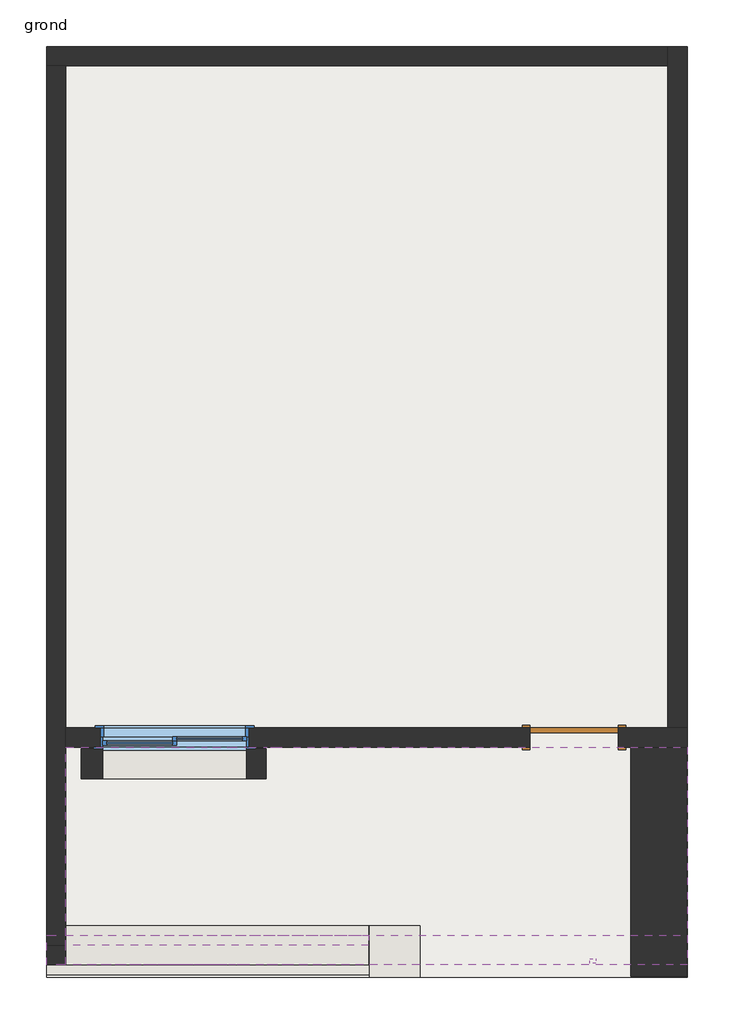
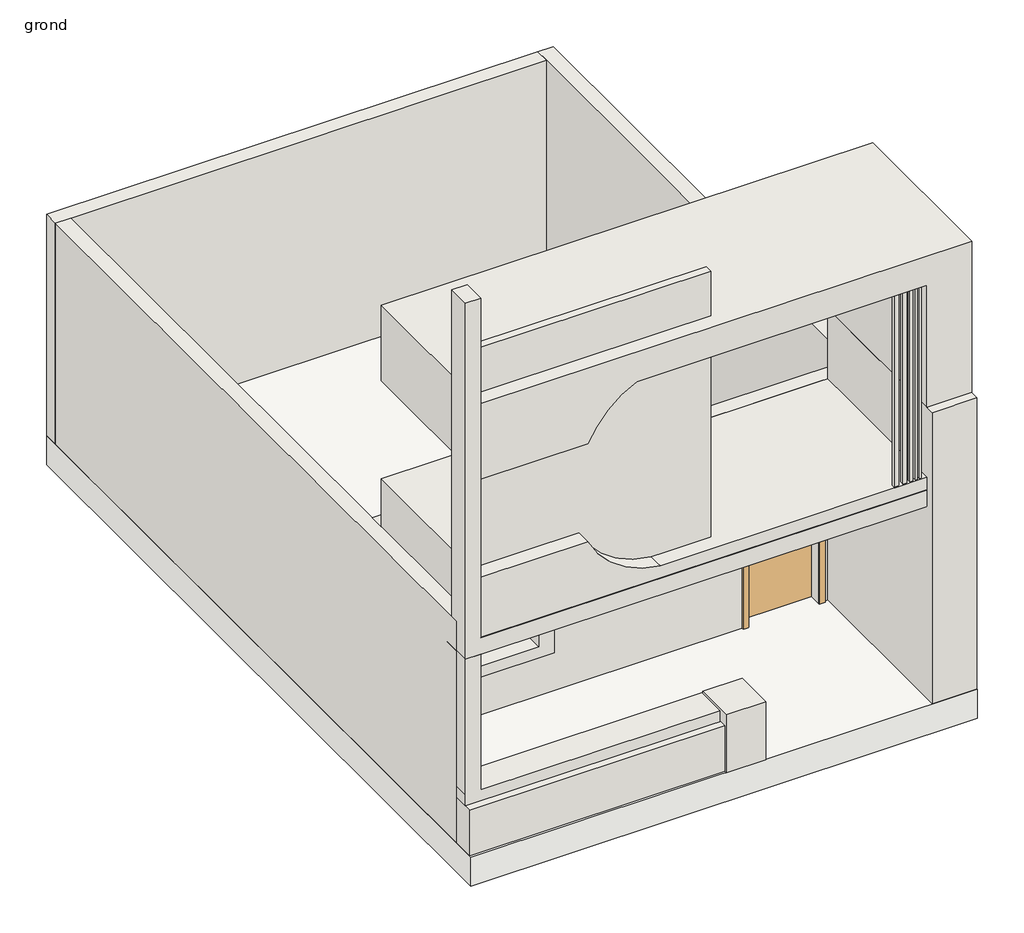
# One storey: 14 walls, 1 door, 1 slab, 1 window.
"""IFC4 building model written with IfcOpenShell, lengths in millimetres."""

from ifc_helpers import new_model, si_unit, frame, origin, origin_with_axes, place, context, project, spatial, polyline, outline, extrude, faceted_brep, transform, mapped, element, save
from components import m_single_flush_0915_x_2134mm_6a9e8738, walls_1_walls_1_6260b2a2, walls_10_walls_10_b49e789a, walls_2_walls_2_db01f069, walls_3_walls_3_21c244ff, walls_4_walls_4_0e46dea8, walls_5_walls_5_5868f2dc, walls_6_walls_6_38c579e2, walls_8_walls_8_e14edf94, walls_9_walls_9_94da1e13, window_c4d7a2b1

model = new_model("IFC4")

# Units and contexts
model_context = context("Model", 3, world=origin())
ifc_project = project(units=[si_unit("LENGTHUNIT", "METRE", prefix="MILLI")], contexts=[model_context])

# Site, building, storey
site = spatial("IfcSite", under=ifc_project)
building = spatial("IfcBuilding", under=site)
storey = spatial("IfcBuildingStorey", under=building, Name="grond", Elevation=0.0)

# Door
placement = place(None, origin())
m_single_flush_0915_x_2134mm_shape = m_single_flush_0915_x_2134mm_6a9e8738(model_context)
element("IfcDoor", 1, ObjectType="M_Single-Flush : 0915 x 2134mm", at=placement, inside=storey, context=model_context, shape_type="MappedRepresentation", body=[
    mapped(m_single_flush_0915_x_2134mm_shape, transform((-7079.0996792, -5453.0913939, 0.0), x_axis=(1.0, 0.0, 0.0), y_axis=(0.0, 1.0, 0.0), z_axis=(0.0, 0.0, 1.0))),
])

# Slab
element("IfcSlab", 2, ObjectType="Generic Floor - 400mm", at=placement, inside=storey, context=model_context, shape_type="SweptSolid", body=[
    extrude(outline(polyline([(-5912.2996792, 1657.3086061), (-5912.2996792, -7921.8501996), (-12513.0996792, -7921.8501996), (-12513.0996792, 1657.3086061), (-5912.2996792, 1657.3086061)])), frame((0.0, 0.0, -400.0), z_axis=(0.0, 0.0, 1.0), x_axis=(1.0, 0.0, 0.0)), (0.0, 0.0, 1.0), 400.0),
])

# Walls
element("IfcWall", 3, ObjectType="Generic - 9\"", at=placement, inside=storey, context=model_context, shape_type="Brep", body=[
    faceted_brep([(-12513.0996792, 1457.3086061, 0.0), (-12313.0996792, 1457.3086061, 0.0), (-6112.2996792, 1457.3086061, 0.0), (-6112.2996792, 1457.3086061, 3048.0), (-12313.0996792, 1457.3086061, 3048.0), (-12513.0996792, 1457.3086061, 3048.0), (-12513.0996792, 1657.3086061, 0.0), (-12513.0996792, 1657.3086061, 3048.0), (-6112.2996792, 1657.3086061, 3048.0), (-6112.2996792, 1657.3086061, 0.0)], [[[0, 1, 2, 3, 4, 5]], [[6, 7, 8, 9]], [[2, 1, 0, 6, 9]], [[5, 4, 3, 8, 7]], [[0, 5, 7, 6]], [[3, 2, 9, 8]]]),
])
element("IfcWall", 4, ObjectType="Generic - 9\"", at=placement, inside=storey, context=model_context, shape_type="Brep", body=[
    faceted_brep([(-12313.0996792, -7590.0501996, 0.0), (-12313.0996792, -7390.0501996, 0.0), (-12313.0996792, -5553.0913939, 0.0), (-12313.0996792, -5353.0913939, 0.0), (-12313.0996792, 1457.3086061, 0.0), (-12313.0996792, 1457.3086061, 3048.0), (-12313.0996792, -5353.0913939, 3048.0), (-12313.0996792, -5553.0913939, 3048.0), (-12313.0996792, -7590.0501996, 3048.0), (-12313.0996792, -7590.0501996, 627.4738057), (-12513.0996792, -7590.0501996, 0.0), (-12513.0996792, -7590.0501996, 3048.0), (-12513.0996792, 1457.3086061, 3048.0), (-12513.0996792, 1457.3086061, 0.0)], [[[0, 1, 2, 3, 4, 5, 6, 7, 8, 9]], [[10, 11, 12, 13]], [[4, 3, 2, 1, 0, 10, 13]], [[8, 7, 6, 5, 12, 11]], [[5, 4, 13, 12]], [[0, 9, 8, 11, 10]]]),
])
element("IfcWall", 5, ObjectType="Generic - 9\"", at=placement, inside=storey, context=model_context, shape_type="Brep", body=[
    faceted_brep([(-5912.2996792, -5353.0913939, 0.0), (-6112.2996792, -5353.0913939, 0.0), (-6621.5996792, -5353.0913939, 0.0), (-6621.5996792, -5353.0913939, 2134.0), (-7536.5996792, -5353.0913939, 2134.0), (-7536.5996792, -5353.0913939, 0.0), (-12313.0996792, -5353.0913939, 0.0), (-12313.0996792, -5353.0913939, 3048.0), (-6112.2996792, -5353.0913939, 3048.0), (-5912.2996792, -5353.0913939, 3048.0), (-11955.8996792, -5353.0913939, 2133.6), (-11955.8996792, -5353.0913939, 914.4), (-10431.8996792, -5353.0913939, 914.4), (-10431.8996792, -5353.0913939, 2133.6), (-6621.5996792, -5553.0913939, 2134.0), (-6621.5996792, -5553.0913939, 0.0), (-5912.2996792, -5553.0913939, 0.0), (-5912.2996792, -5553.0913939, 3048.0), (-12313.0996792, -5553.0913939, 3048.0), (-12313.0996792, -5553.0913939, 0.0), (-7536.5996792, -5553.0913939, 0.0), (-7536.5996792, -5553.0913939, 2134.0), (-11955.8996792, -5553.0913939, 2133.6), (-10431.8996792, -5553.0913939, 2133.6), (-10431.8996792, -5553.0913939, 914.4), (-11955.8996792, -5553.0913939, 914.4)], [[[0, 1, 2, 3, 4, 5, 6, 7, 8, 9], [10, 11, 12, 13]], [[14, 15, 16, 17, 18, 19, 20, 21], [22, 23, 24, 25]], [[20, 19, 6, 5]], [[16, 15, 2, 1, 0]], [[9, 8, 7, 18, 17]], [[0, 9, 17, 16]], [[3, 2, 15, 14]], [[4, 3, 14, 21]], [[5, 4, 21, 20]], [[11, 10, 22, 25]], [[12, 11, 25, 24]], [[13, 12, 24, 23]], [[10, 13, 23, 22]], [[7, 6, 19, 18]]]),
])
element("IfcWall", 6, ObjectType="Generic - 9\"", at=placement, inside=storey, context=model_context, shape_type="Brep", body=[
    faceted_brep([(-6112.2996792, 1657.3086061, 0.0), (-6112.2996792, 1457.3086061, 0.0), (-6112.2996792, -5353.0913939, 0.0), (-6112.2996792, -5353.0913939, 3048.0), (-6112.2996792, 1457.3086061, 3048.0), (-6112.2996792, 1657.3086061, 3048.0), (-5912.2996792, 1657.3086061, 0.0), (-5912.2996792, 1657.3086061, 3048.0), (-5912.2996792, -5353.0913939, 3048.0), (-5912.2996792, -5353.0913939, 0.0)], [[[0, 1, 2, 3, 4, 5]], [[6, 7, 8, 9]], [[2, 1, 0, 6, 9]], [[5, 4, 3, 8, 7]], [[0, 5, 7, 6]], [[3, 2, 9, 8]]]),
])
element("IfcWall", 7, ObjectType="Generic - 9\"", at=placement, inside=storey, context=model_context, shape_type="SweptSolid", body=[
    extrude(outline(polyline([(-9187.2996792, -7590.0501996), (-12313.0996792, -7590.0501996), (-12313.0996792, -7390.0501996), (-9187.2996792, -7390.0501996), (-9187.2996792, -7590.0501996)])), origin_with_axes(), (0.0, 0.0, 1.0), 627.4738057),
])
walls_1_walls_1_shape = walls_1_walls_1_6260b2a2(model_context)
element("IfcWall", 8, ObjectType="Walls 1 : Walls 1", at=placement, inside=storey, context=model_context, shape_type="MappedRepresentation", body=[
    mapped(walls_1_walls_1_shape, transform((0.0, 0.0, 0.0), x_axis=(1.0, 0.0, 0.0), y_axis=(0.0, 1.0, 0.0), z_axis=(0.0, 0.0, 1.0))),
])
walls_10_walls_10_shape = walls_10_walls_10_b49e789a(model_context)
element("IfcWall", 9, ObjectType="Walls 10 : Walls 10", at=placement, inside=storey, context=model_context, shape_type="MappedRepresentation", body=[
    mapped(walls_10_walls_10_shape, transform((0.0, 0.0, 0.0), x_axis=(1.0, 0.0, 0.0), y_axis=(0.0, 1.0, 0.0), z_axis=(0.0, 0.0, 1.0))),
])
walls_2_walls_2_shape = walls_2_walls_2_db01f069(model_context)
element("IfcWall", 10, ObjectType="Walls 2 : Walls 2", at=placement, inside=storey, context=model_context, shape_type="MappedRepresentation", body=[
    mapped(walls_2_walls_2_shape, transform((0.0, 0.0, 0.0), x_axis=(1.0, 0.0, 0.0), y_axis=(0.0, 1.0, 0.0), z_axis=(0.0, 0.0, 1.0))),
])
walls_3_walls_3_shape = walls_3_walls_3_21c244ff(model_context)
element("IfcWall", 11, ObjectType="Walls 3 : Walls 3", at=placement, inside=storey, context=model_context, shape_type="MappedRepresentation", body=[
    mapped(walls_3_walls_3_shape, transform((0.0, 0.0, 0.0), x_axis=(1.0, 0.0, 0.0), y_axis=(0.0, 1.0, 0.0), z_axis=(0.0, 0.0, 1.0))),
])
walls_4_walls_4_shape = walls_4_walls_4_0e46dea8(model_context)
element("IfcWall", 12, ObjectType="Walls 4 : Walls 4", at=placement, inside=storey, context=model_context, shape_type="MappedRepresentation", body=[
    mapped(walls_4_walls_4_shape, transform((0.0, 0.0, 0.0), x_axis=(1.0, 0.0, 0.0), y_axis=(0.0, 1.0, 0.0), z_axis=(0.0, 0.0, 1.0))),
])
walls_5_walls_5_shape = walls_5_walls_5_5868f2dc(model_context)
element("IfcWall", 13, ObjectType="Walls 5 : Walls 5", at=placement, inside=storey, context=model_context, shape_type="MappedRepresentation", body=[
    mapped(walls_5_walls_5_shape, transform((0.0, 0.0, 0.0), x_axis=(1.0, 0.0, 0.0), y_axis=(0.0, 1.0, 0.0), z_axis=(0.0, 0.0, 1.0))),
])
walls_6_walls_6_shape = walls_6_walls_6_38c579e2(model_context)
element("IfcWall", 14, ObjectType="Walls 6 : Walls 6", at=placement, inside=storey, context=model_context, shape_type="MappedRepresentation", body=[
    mapped(walls_6_walls_6_shape, transform((0.0, 0.0, 0.0), x_axis=(1.0, 0.0, 0.0), y_axis=(0.0, 1.0, 0.0), z_axis=(0.0, 0.0, 1.0))),
])
walls_8_walls_8_shape = walls_8_walls_8_e14edf94(model_context)
element("IfcWall", 15, ObjectType="Walls 8 : Walls 8", at=placement, inside=storey, context=model_context, shape_type="MappedRepresentation", body=[
    mapped(walls_8_walls_8_shape, transform((103.6381573, 0.0, -6.9092105), x_axis=(1.0, 0.0, 0.0), y_axis=(0.0, 1.0, 0.0), z_axis=(0.0, 0.0, 1.0))),
])
walls_9_walls_9_shape = walls_9_walls_9_94da1e13(model_context)
element("IfcWall", 16, ObjectType="Walls 9 : Walls 9", at=placement, inside=storey, context=model_context, shape_type="MappedRepresentation", body=[
    mapped(walls_9_walls_9_shape, transform((0.0, 0.0, 0.0), x_axis=(1.0, 0.0, 0.0), y_axis=(0.0, 1.0, 0.0), z_axis=(0.0, 0.0, 1.0))),
])

# Window
window_shape = window_c4d7a2b1(model_context)
element("IfcWindow", 17, ObjectType="Slider with Trim : 60\" x 48\"", at=placement, inside=storey, context=model_context, shape_type="MappedRepresentation", body=[
    mapped(window_shape, transform((-11193.8996792, -5453.0913939, 0.0), x_axis=(-1.0, 0.0, 0.0), y_axis=(0.0, -1.0, 0.0), z_axis=(0.0, 0.0, 1.0))),
])

save(model, "model.ifc")

# Revit data of these elements
# Type "M_Single-Flush : 0915 x 2134mm"
#   Type Mark = "15"
#   Thickness = 51 mm
#   Height = 2134 mm
#   Trim Projection Ext = 25 mm
#   Trim Projection Int = 25 mm
#   Trim Width = 76 mm
#   Width = 915 mm
#   Door Material = Door - Panel
#   Frame Material = Door - Frame
#   Function = (empty or 0)
#   Wall Closure = (empty or 0)
# Type "Generic Floor - 400mm"
#   Function = 0
#   Layers, outside or top first: 400 mm no material (function 1)
# Type "Generic - 9\""
#   Layers, outside or top first: 200 mm no material (function 1)
# Type "Slider with Trim : 60\" x 48\""
#   Type Mark = "22"
#   Construction Type Id = "GSP4R"
#   Assembly Code = "B2020100"
#   Analytic Construction = "1/8 in Pilkington single glazing"
#   Visual Light Transmittance = 0.9
#   Solar Heat Gain Coefficient = 0.78
#   Heat Transfer Coefficient (U) = 3.6886 W/(m²·K)
#   Height = 1219.2 mm
#   Default Sill Height = 914.4 mm
#   Trim Projection - Ext. = 19.05 mm
#   Trim Projection - Int. = 19.05 mm
#   Trim Width - Exterior = 88.9 mm
#   Trim Width - Interior = 88.9 mm
#   Width = 1524 mm
#   Window Inset = 19.05 mm
#   Define Thermal Properties by = 1
#   Glass Pane Material = Glass
#   Sash Material = Sash
#   Trim Exterior Material = Trim
#   Trim Interior Material = Trim
#   Wall Closure = (empty or 0)
# Element 1 (IfcDoor, "M_Single-Flush : 0915 x 2134mm")
#   Phase Created = New Construction
#   Materials on its faces: "Door - Frame", "Door - Panel"
# Element 2 (IfcSlab, "Generic Floor - 400mm")
#   Height Offset From Level = 0 mm
#   Phase Created = New Construction
#   Materials on its faces: "Default Roof"
# Elements 3, 4, 5, 6 (IfcWall, "Generic - 9\"")
#   Top Offset = 0 mm
#   Base Offset = 0 mm
#   Unconnected Height = 3048 mm
#   wall height = 3048 mm
#   Phase Created = New Construction
#   Base Constraint = grond
#   Materials on its faces: "Default Wall"
# Element 7 (IfcWall, "Generic - 9\"")
#   Top Offset = 0 mm
#   Base Offset = 0 mm
#   Unconnected Height = 627.474 mm
#   wall height = 627.474 mm
#   Phase Created = New Construction
#   Base Constraint = grond
#   Materials on its faces: "Default Wall"
# Element 8 (IfcWall, "Walls 1 : Walls 1")
#   Phase Created = New Construction
#   Materials on its faces: "Default Wall"
# Element 9 (IfcWall, "Walls 10 : Walls 10")
#   Phase Created = New Construction
#   Materials on its faces: "Default Wall"
# Element 10 (IfcWall, "Walls 2 : Walls 2")
#   Phase Created = New Construction
#   Materials on its faces: "Default Wall"
# Element 11 (IfcWall, "Walls 3 : Walls 3")
#   Phase Created = New Construction
#   Materials on its faces: "Default Wall"
# Element 12 (IfcWall, "Walls 4 : Walls 4")
#   Phase Created = New Construction
#   Materials on its faces: "Default Wall"
# Element 13 (IfcWall, "Walls 5 : Walls 5")
#   Phase Created = New Construction
#   Materials on its faces: "Default Wall"
# Element 14 (IfcWall, "Walls 6 : Walls 6")
#   Phase Created = New Construction
#   Materials on its faces: "Default Wall"
# Element 15 (IfcWall, "Walls 8 : Walls 8")
#   Phase Created = New Construction
#   Materials on its faces: "Default Wall"
# Element 16 (IfcWall, "Walls 9 : Walls 9")
#   Phase Created = New Construction
#   Materials on its faces: "Default Wall"
# Element 17 (IfcWindow, "Slider with Trim : 60\" x 48\"")
#   Mark = "7"
#   Phase Created = New Construction
#   Materials on its faces: "Sash", "Trim", "Glass"
# Materials
#   "Door - Panel": class "Wood", colour RGB 114 82 51, transparency 0
#   "Door - Frame": colour RGB 153 76 43, transparency 0
#   "Glass": class "Glass", colour RGB 218 227 224, transparency 0.85, Description = "Soda Lime Glass", Cost = 0
#   "Sash": class "Wood", colour RGB 136 99 55, transparency 0
#   "Trim": class "Wood", colour RGB 224 178 126, transparency 0
#   "Default Roof": colour RGB 80 80 80, transparency 0
#   "Default Wall": colour RGB 80 80 80, transparency 0
